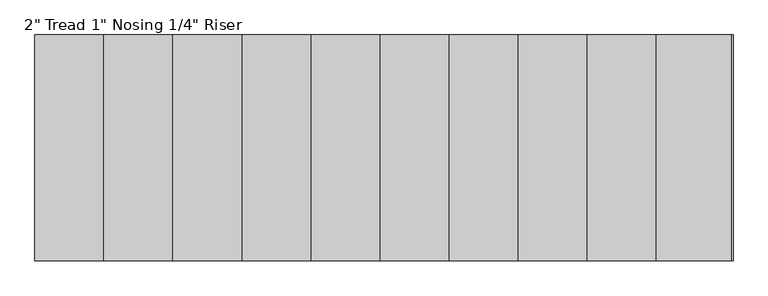
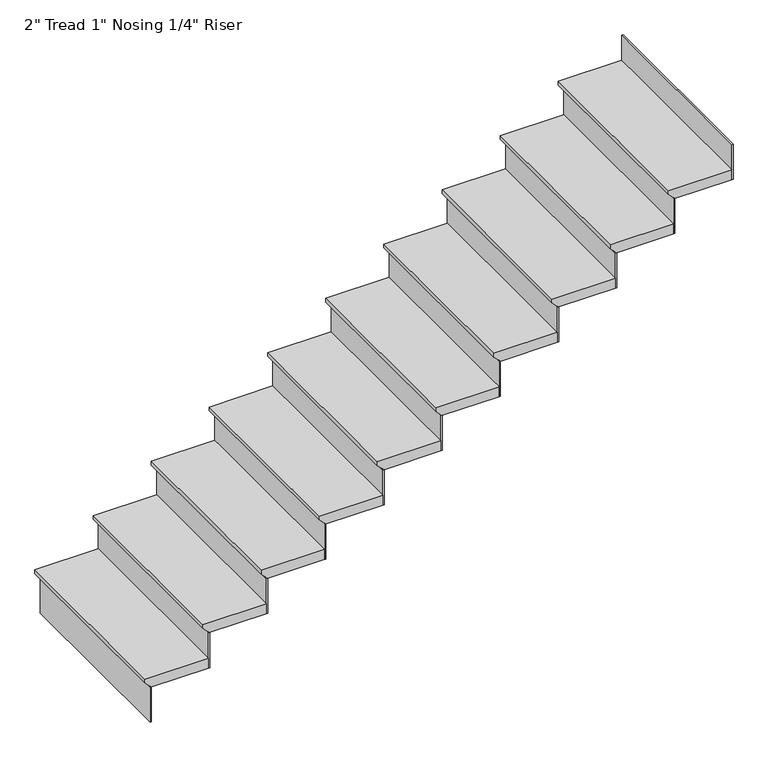
"""IFC4 building model written with IfcOpenShell, lengths in millimetres: stair flight geometry."""

from ifc_helpers import new_model, si_unit, frame, origin, place, context, project, spatial, polyline, outline, extrude, source, transform, mapped, element, save


def stair_flight_c36fe085(model_context):
    return source(origin(), model_context, "Body", "SweptSolid", [
        extrude(outline(polyline([(4622.8, -12010.1954771), (4622.8, -12314.9954771), (4603.75, -12314.9954771), (4578.35, -12289.5954771), (4572.0, -12289.5954771), (4572.0, -12010.1954771), (4622.8, -12010.1954771)])), frame((0.0, 2764.4129676, 0.0), z_axis=(0.0, 1.0, 0.0), x_axis=(0.0, 0.0, 1.0)), (0.0, 0.0, 1.0), 914.4),
        extrude(outline(polyline([(-12283.2454771, 2764.4129676), (-12289.5954771, 2764.4129676), (-12289.5954771, 3678.8129676), (-12283.2454771, 3678.8129676), (-12283.2454771, 2764.4129676)])), frame((0.0, 0.0, 4394.2), z_axis=(0.0, 0.0, 1.0), x_axis=(1.0, 0.0, 0.0)), (0.0, 0.0, 1.0), 177.8),
        extrude(outline(polyline([(-12003.8454771, 2764.4129676), (-12010.1954771, 2764.4129676), (-12010.1954771, 3678.8129676), (-12003.8454771, 3678.8129676), (-12003.8454771, 2764.4129676)])), frame((0.0, 0.0, 4572.0), z_axis=(0.0, 0.0, 1.0), x_axis=(1.0, 0.0, 0.0)), (0.0, 0.0, 1.0), 177.8),
        extrude(outline(polyline([(4800.6, -11730.7954771), (4800.6, -12035.5954771), (4781.55, -12035.5954771), (4756.15, -12010.1954771), (4749.8, -12010.1954771), (4749.8, -11730.7954771), (4800.6, -11730.7954771)])), frame((0.0, 2764.4129676, 0.0), z_axis=(0.0, 1.0, 0.0), x_axis=(0.0, 0.0, 1.0)), (0.0, 0.0, 1.0), 914.4),
        extrude(outline(polyline([(-11724.4454771, 2764.4129676), (-11730.7954771, 2764.4129676), (-11730.7954771, 3678.8129676), (-11724.4454771, 3678.8129676), (-11724.4454771, 2764.4129676)])), frame((0.0, 0.0, 4749.8), z_axis=(0.0, 0.0, 1.0), x_axis=(1.0, 0.0, 0.0)), (0.0, 0.0, 1.0), 177.8),
        extrude(outline(polyline([(4978.4, -11451.3954771), (4978.4, -11756.1954771), (4959.35, -11756.1954771), (4933.95, -11730.7954771), (4927.6, -11730.7954771), (4927.6, -11451.3954771), (4978.4, -11451.3954771)])), frame((0.0, 2764.4129676, 0.0), z_axis=(0.0, 1.0, 0.0), x_axis=(0.0, 0.0, 1.0)), (0.0, 0.0, 1.0), 914.4),
        extrude(outline(polyline([(-11445.0454771, 2764.4129676), (-11451.3954771, 2764.4129676), (-11451.3954771, 3678.8129676), (-11445.0454771, 3678.8129676), (-11445.0454771, 2764.4129676)])), frame((0.0, 0.0, 4927.6), z_axis=(0.0, 0.0, 1.0), x_axis=(1.0, 0.0, 0.0)), (0.0, 0.0, 1.0), 177.8),
        extrude(outline(polyline([(5156.2, -11171.9954771), (5156.2, -11476.7954771), (5137.15, -11476.7954771), (5111.75, -11451.3954771), (5105.4, -11451.3954771), (5105.4, -11171.9954771), (5156.2, -11171.9954771)])), frame((0.0, 2764.4129676, 0.0), z_axis=(0.0, 1.0, 0.0), x_axis=(0.0, 0.0, 1.0)), (0.0, 0.0, 1.0), 914.4),
        extrude(outline(polyline([(-11165.6454771, 2764.4129676), (-11171.9954771, 2764.4129676), (-11171.9954771, 3678.8129676), (-11165.6454771, 3678.8129676), (-11165.6454771, 2764.4129676)])), frame((0.0, 0.0, 5105.4), z_axis=(0.0, 0.0, 1.0), x_axis=(1.0, 0.0, 0.0)), (0.0, 0.0, 1.0), 177.8),
        extrude(outline(polyline([(5334.0, -10892.5954771), (5334.0, -11197.3954771), (5314.95, -11197.3954771), (5289.55, -11171.9954771), (5283.2, -11171.9954771), (5283.2, -10892.5954771), (5334.0, -10892.5954771)])), frame((0.0, 2764.4129676, 0.0), z_axis=(0.0, 1.0, 0.0), x_axis=(0.0, 0.0, 1.0)), (0.0, 0.0, 1.0), 914.4),
        extrude(outline(polyline([(-10886.2454771, 2764.4129676), (-10892.5954771, 2764.4129676), (-10892.5954771, 3678.8129676), (-10886.2454771, 3678.8129676), (-10886.2454771, 2764.4129676)])), frame((0.0, 0.0, 5283.2), z_axis=(0.0, 0.0, 1.0), x_axis=(1.0, 0.0, 0.0)), (0.0, 0.0, 1.0), 177.8),
        extrude(outline(polyline([(5511.8, -10613.1954771), (5511.8, -10917.9954771), (5492.75, -10917.9954771), (5467.35, -10892.5954771), (5461.0, -10892.5954771), (5461.0, -10613.1954771), (5511.8, -10613.1954771)])), frame((0.0, 2764.4129676, 0.0), z_axis=(0.0, 1.0, 0.0), x_axis=(0.0, 0.0, 1.0)), (0.0, 0.0, 1.0), 914.4),
        extrude(outline(polyline([(-10606.8454771, 2764.4129676), (-10613.1954771, 2764.4129676), (-10613.1954771, 3678.8129676), (-10606.8454771, 3678.8129676), (-10606.8454771, 2764.4129676)])), frame((0.0, 0.0, 5461.0), z_axis=(0.0, 0.0, 1.0), x_axis=(1.0, 0.0, 0.0)), (0.0, 0.0, 1.0), 177.8),
        extrude(outline(polyline([(5689.6, -10333.7954771), (5689.6, -10638.5954771), (5670.55, -10638.5954771), (5645.15, -10613.1954771), (5638.8, -10613.1954771), (5638.8, -10333.7954771), (5689.6, -10333.7954771)])), frame((0.0, 2764.4129676, 0.0), z_axis=(0.0, 1.0, 0.0), x_axis=(0.0, 0.0, 1.0)), (0.0, 0.0, 1.0), 914.4),
        extrude(outline(polyline([(-10327.4454771, 2764.4129676), (-10333.7954771, 2764.4129676), (-10333.7954771, 3678.8129676), (-10327.4454771, 3678.8129676), (-10327.4454771, 2764.4129676)])), frame((0.0, 0.0, 5638.8), z_axis=(0.0, 0.0, 1.0), x_axis=(1.0, 0.0, 0.0)), (0.0, 0.0, 1.0), 177.8),
        extrude(outline(polyline([(5867.4, -10054.3954771), (5867.4, -10359.1954771), (5848.35, -10359.1954771), (5822.95, -10333.7954771), (5816.6, -10333.7954771), (5816.6, -10054.3954771), (5867.4, -10054.3954771)])), frame((0.0, 2764.4129676, 0.0), z_axis=(0.0, 1.0, 0.0), x_axis=(0.0, 0.0, 1.0)), (0.0, 0.0, 1.0), 914.4),
        extrude(outline(polyline([(-10048.0454771, 2764.4129676), (-10054.3954771, 2764.4129676), (-10054.3954771, 3678.8129676), (-10048.0454771, 3678.8129676), (-10048.0454771, 2764.4129676)])), frame((0.0, 0.0, 5816.6), z_axis=(0.0, 0.0, 1.0), x_axis=(1.0, 0.0, 0.0)), (0.0, 0.0, 1.0), 177.8),
        extrude(outline(polyline([(6045.2, -9774.9954771), (6045.2, -10079.7954771), (6026.15, -10079.7954771), (6000.75, -10054.3954771), (5994.4, -10054.3954771), (5994.4, -9774.9954771), (6045.2, -9774.9954771)])), frame((0.0, 2764.4129676, 0.0), z_axis=(0.0, 1.0, 0.0), x_axis=(0.0, 0.0, 1.0)), (0.0, 0.0, 1.0), 914.4),
        extrude(outline(polyline([(-9768.6454771, 2764.4129676), (-9774.9954771, 2764.4129676), (-9774.9954771, 3678.8129676), (-9768.6454771, 3678.8129676), (-9768.6454771, 2764.4129676)])), frame((0.0, 0.0, 5994.4), z_axis=(0.0, 0.0, 1.0), x_axis=(1.0, 0.0, 0.0)), (0.0, 0.0, 1.0), 177.8),
        extrude(outline(polyline([(-9489.2454771, 2764.4129676), (-9495.5954771, 2764.4129676), (-9495.5954771, 3678.8129676), (-9489.2454771, 3678.8129676), (-9489.2454771, 2764.4129676)])), frame((0.0, 0.0, 6172.2), z_axis=(0.0, 0.0, 1.0), x_axis=(1.0, 0.0, 0.0)), (0.0, 0.0, 1.0), 177.8),
        extrude(outline(polyline([(6223.0, -9495.5954771), (6223.0, -9800.3954771), (6203.95, -9800.3954771), (6178.55, -9774.9954771), (6172.2, -9774.9954771), (6172.2, -9495.5954771), (6223.0, -9495.5954771)])), frame((0.0, 2764.4129676, 0.0), z_axis=(0.0, 1.0, 0.0), x_axis=(0.0, 0.0, 1.0)), (0.0, 0.0, 1.0), 914.4),
    ])


if __name__ == "__main__":
    model = new_model("IFC4")
    model_context = context("Model", 3, world=origin())
    ifc_project = project(units=[si_unit("LENGTHUNIT", "METRE", prefix="MILLI")], contexts=[model_context])
    site = spatial("IfcSite", under=ifc_project)
    building = spatial("IfcBuilding", under=site)
    placement = place(None, origin())
    stair_flight_shape = stair_flight_c36fe085(model_context)
    element("IfcStairFlight", 1, ObjectType="2\" Tread 1\" Nosing 1/4\" Riser", at=placement, inside=building, context=model_context, shape_type="MappedRepresentation", body=[
        mapped(stair_flight_shape, transform((0.0, 0.0, 0.0), x_axis=(1.0, 0.0, 0.0), y_axis=(0.0, 1.0, 0.0), z_axis=(0.0, 0.0, 1.0))),
    ])
    save(model, "model.ifc")
